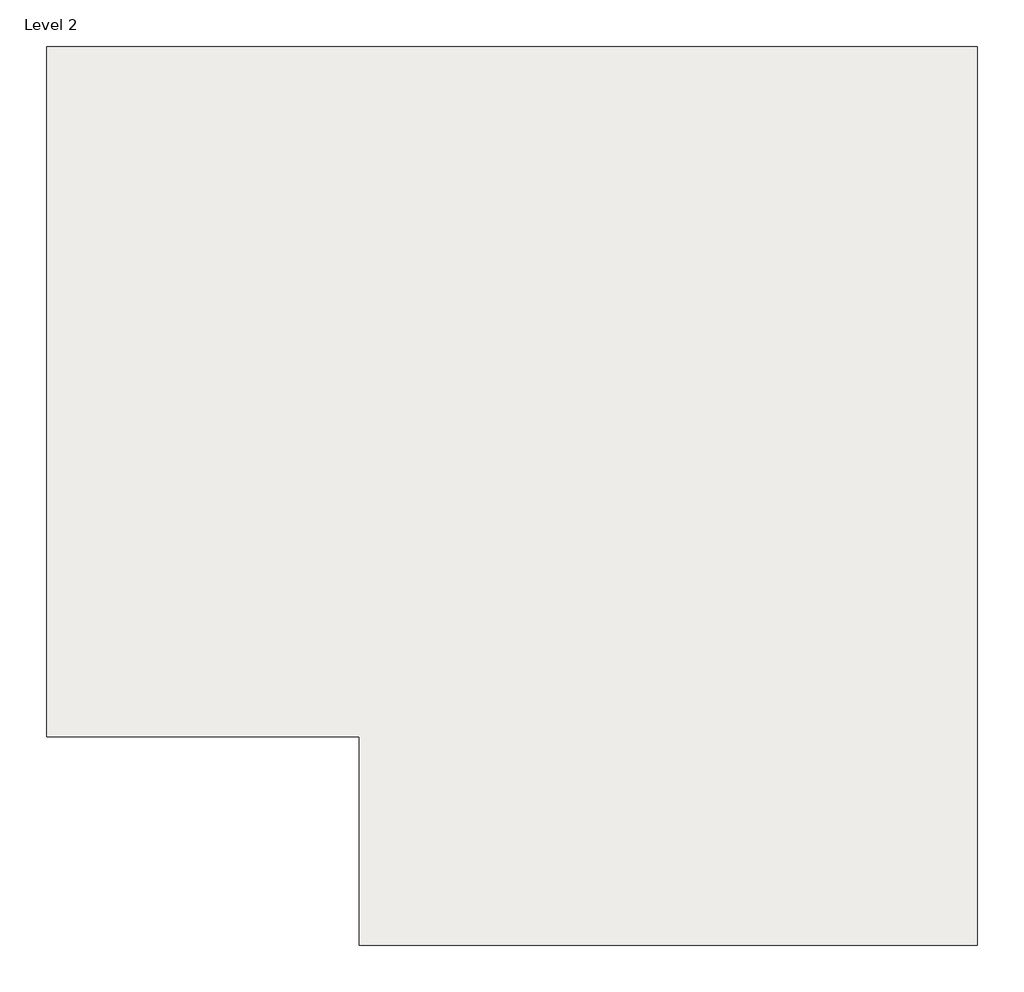
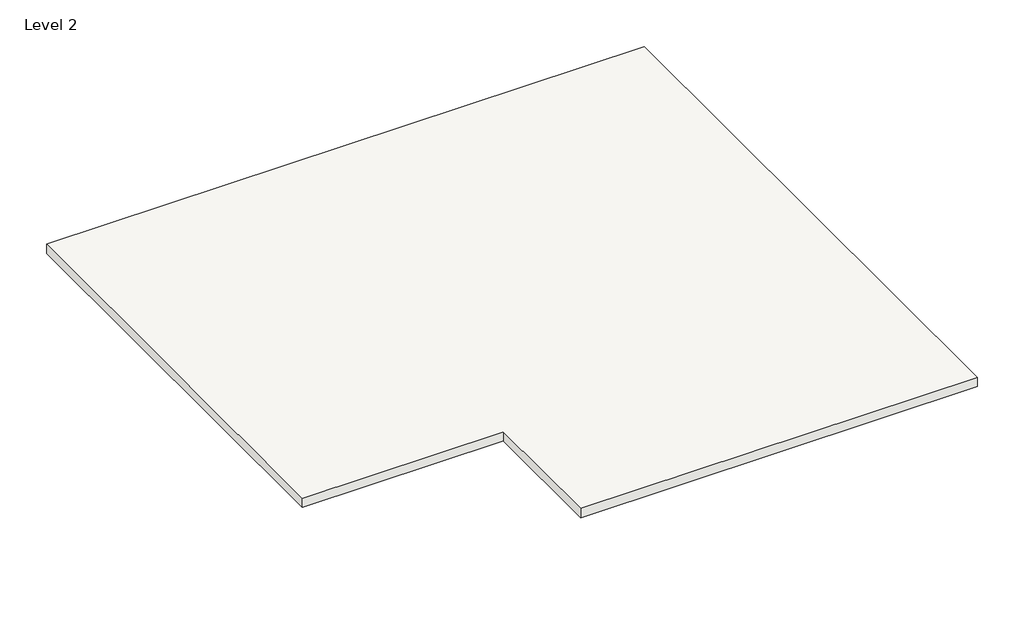
# One storey: 1 roof.
"""IFC4 building model written with IfcOpenShell, lengths in millimetres."""

from ifc_helpers import new_model, si_unit, frame, origin, place, context, project, spatial, polyline, outline, extrude, element, save

model = new_model("IFC4")

# Units and contexts
model_context = context("Model", 3, world=origin())
ifc_project = project(units=[si_unit("LENGTHUNIT", "METRE", prefix="MILLI")], contexts=[model_context])

# Site, building, storey
site = spatial("IfcSite", under=ifc_project)
building = spatial("IfcBuilding", under=site)
storey = spatial("IfcBuildingStorey", under=building, Name="Level 2", Elevation=3048.0)

# Roof
placement = place(None, origin())
element("IfcRoof", 1, ObjectType="6\"", at=placement, inside=storey, context=model_context, shape_type="SweptSolid", body=[
    extrude(outline(polyline([(-8080.8102438, -2410.8934581), (-11281.2102438, -2410.8934581), (-11281.2102438, 4650.3065419), (-1756.2102438, 4650.3065419), (-1756.2102438, -4544.4934581), (-8080.8102438, -4544.4934581), (-8080.8102438, -2410.8934581)])), frame((0.0, 0.0, 3048.0), z_axis=(0.0, 0.0, 1.0), x_axis=(1.0, 0.0, 0.0)), (0.0, 0.0, 1.0), 152.4),
])

save(model, "model.ifc")

# Revit data of these elements
# Type "6\""
#   Assembly Code = "B1020"
#   Layers, outside or top first: 0' - 6" "Gypsum Wall Board" (function 1)
# Element 1 (IfcRoof, "6\"")
#   built-in parameter 1001705 = 10.5 (stored number, unit not read)
#   built-in parameter 1001710 = 33615
#   Phase Created = New Construction
#   Materials on its faces: "Gypsum Wall Board"
# Materials
#   "Gypsum Wall Board": class "Generic", colour RGB 127 127 127, transparency 0, Description = "Gypsum Wall Board", Cost = 0
